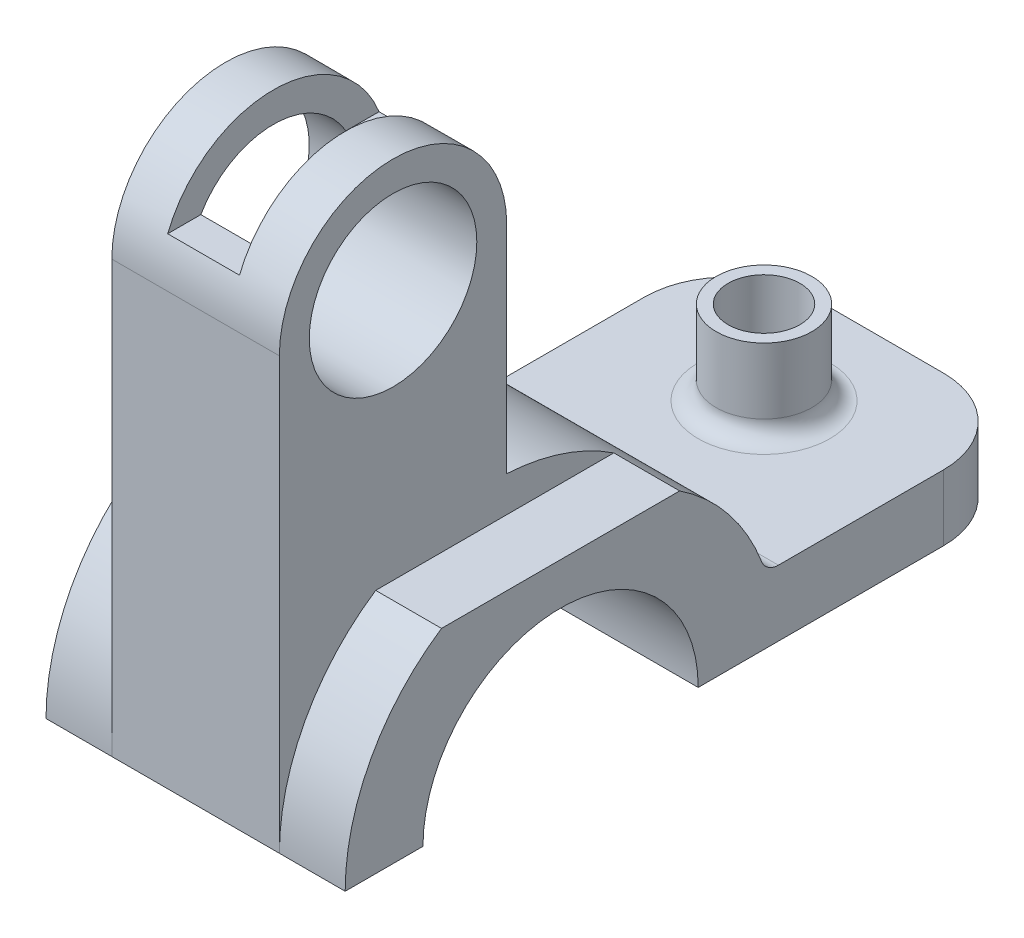
ISO-10303-21;
HEADER;
FILE_DESCRIPTION(('STEP AP214'),'2;1');
FILE_NAME('part.step','',(''),(''),'','','');
FILE_SCHEMA(('AUTOMOTIVE_DESIGN { 1 0 10303 214 1 1 1 1 }'));
ENDSEC;
DATA;
#1=APPLICATION_CONTEXT('core data for automotive mechanical design processes');
#2=APPLICATION_PROTOCOL_DEFINITION('international standard','automotive_design',2000,#1);
#3=PRODUCT_CONTEXT('',#1,'mechanical');
#4=PRODUCT('Part','Part','',(#3));
#5=PRODUCT_RELATED_PRODUCT_CATEGORY('part','',(#4));
#6=PRODUCT_DEFINITION_FORMATION('','',#4);
#7=PRODUCT_DEFINITION_CONTEXT('part definition',#1,'design');
#8=PRODUCT_DEFINITION('design','',#6,#7);
#9=PRODUCT_DEFINITION_SHAPE('','',#8);
#10=(LENGTH_UNIT() NAMED_UNIT(*) SI_UNIT(.MILLI.,.METRE.));
#11=(NAMED_UNIT(*) PLANE_ANGLE_UNIT() SI_UNIT($,.RADIAN.));
#12=(NAMED_UNIT(*) SI_UNIT($,.STERADIAN.) SOLID_ANGLE_UNIT());
#13=UNCERTAINTY_MEASURE_WITH_UNIT(LENGTH_MEASURE(1.E-05),#10,'distance_accuracy_value','');
#14=(GEOMETRIC_REPRESENTATION_CONTEXT(3) GLOBAL_UNCERTAINTY_ASSIGNED_CONTEXT((#13)) GLOBAL_UNIT_ASSIGNED_CONTEXT((#10,
#11,#12)) REPRESENTATION_CONTEXT('',''));
#15=CARTESIAN_POINT('',(0.,0.,0.));
#16=DIRECTION('',(0.,0.,1.));
#17=DIRECTION('',(1.,0.,0.));
#18=AXIS2_PLACEMENT_3D('',#15,#16,#17);
#19=CARTESIAN_POINT('',(14.,72.,17.));
#20=DIRECTION('',(-1.,0.,0.));
#21=DIRECTION('',(0.,0.,1.));
#22=AXIS2_PLACEMENT_3D('',#19,#20,#21);
#23=CYLINDRICAL_SURFACE('',#22,19.);
#24=CARTESIAN_POINT('',(14.,72.,17.));
#25=DIRECTION('',(1.,0.,0.));
#26=DIRECTION('',(0.,0.,-1.));
#27=AXIS2_PLACEMENT_3D('',#24,#25,#26);
#28=CIRCLE('',#27,19.);
#29=CARTESIAN_POINT('',(14.,72.,-1.99999999999999));
#30=VERTEX_POINT('',#29);
#31=CARTESIAN_POINT('',(14.,72.,36.));
#32=VERTEX_POINT('',#31);
#33=EDGE_CURVE('E308',#30,#32,#28,.T.);
#34=ORIENTED_EDGE('',*,*,#33,.F.);
#35=DIRECTION('',(-1.,0.,0.));
#36=VECTOR('',#35,1.);
#37=CARTESIAN_POINT('',(14.,72.,-1.99999999999999));
#38=LINE('',#37,#36);
#39=CARTESIAN_POINT('',(-14.,72.,-1.99999999999999));
#40=VERTEX_POINT('',#39);
#41=EDGE_CURVE('E288',#30,#40,#38,.T.);
#42=ORIENTED_EDGE('',*,*,#41,.T.);
#43=CARTESIAN_POINT('',(-14.,72.,17.));
#44=DIRECTION('',(1.,0.,0.));
#45=DIRECTION('',(0.,0.,-1.));
#46=AXIS2_PLACEMENT_3D('',#43,#44,#45);
#47=CIRCLE('',#46,19.);
#48=CARTESIAN_POINT('',(-14.,72.,36.));
#49=VERTEX_POINT('',#48);
#50=EDGE_CURVE('E314',#40,#49,#47,.T.);
#51=ORIENTED_EDGE('',*,*,#50,.T.);
#52=DIRECTION('',(-1.,0.,0.));
#53=VECTOR('',#52,1.);
#54=CARTESIAN_POINT('',(14.,72.,36.));
#55=LINE('',#54,#53);
#56=EDGE_CURVE('E293',#32,#49,#55,.T.);
#57=ORIENTED_EDGE('',*,*,#56,.F.);
#58=EDGE_LOOP('',(#34,#42,#51,#57));
#59=FACE_BOUND('',#58,.T.);
#60=CARTESIAN_POINT('',(-6.,72.,17.));
#61=DIRECTION('',(1.,0.,0.));
#62=DIRECTION('',(0.,0.,-1.));
#63=AXIS2_PLACEMENT_3D('',#60,#61,#62);
#64=CIRCLE('',#63,19.);
#65=CARTESIAN_POINT('',(-6.,78.9999999999999,-0.663521732655735));
#66=VERTEX_POINT('',#65);
#67=CARTESIAN_POINT('',(-6.,78.9999999999997,34.6635217326558));
#68=VERTEX_POINT('',#67);
#69=EDGE_CURVE('E53',#66,#68,#64,.T.);
#70=ORIENTED_EDGE('',*,*,#69,.F.);
#71=DIRECTION('',(-1.,0.,0.));
#72=VECTOR('',#71,1.);
#73=CARTESIAN_POINT('',(14.,78.9999999999999,-0.663521732655735));
#74=LINE('',#73,#72);
#75=CARTESIAN_POINT('',(6.,78.9999999999999,-0.663521732655735));
#76=VERTEX_POINT('',#75);
#77=EDGE_CURVE('E354',#76,#66,#74,.T.);
#78=ORIENTED_EDGE('',*,*,#77,.F.);
#79=CARTESIAN_POINT('',(6.,72.,17.));
#80=DIRECTION('',(-1.,0.,0.));
#81=DIRECTION('',(0.,0.,1.));
#82=AXIS2_PLACEMENT_3D('',#79,#80,#81);
#83=CIRCLE('',#82,19.);
#84=CARTESIAN_POINT('',(6.,78.9999999999997,34.6635217326558));
#85=VERTEX_POINT('',#84);
#86=EDGE_CURVE('E348',#85,#76,#83,.T.);
#87=ORIENTED_EDGE('',*,*,#86,.F.);
#88=DIRECTION('',(-1.,0.,0.));
#89=VECTOR('',#88,1.);
#90=CARTESIAN_POINT('',(14.,78.9999999999997,34.6635217326558));
#91=LINE('',#90,#89);
#92=EDGE_CURVE('E355',#68,#85,#91,.F.);
#93=ORIENTED_EDGE('',*,*,#92,.F.);
#94=EDGE_LOOP('',(#70,#78,#87,#93));
#95=FACE_BOUND('',#94,.T.);
#96=ADVANCED_FACE('F39',(#59,#95),#23,.T.);
#97=CARTESIAN_POINT('',(25.,72.,17.));
#98=DIRECTION('',(-1.,0.,0.));
#99=DIRECTION('',(0.,0.,1.));
#100=AXIS2_PLACEMENT_3D('',#97,#98,#99);
#101=CYLINDRICAL_SURFACE('',#100,14.);
#102=CARTESIAN_POINT('',(-14.,72.,17.));
#103=DIRECTION('',(-1.,0.,0.));
#104=DIRECTION('',(0.,0.,1.));
#105=AXIS2_PLACEMENT_3D('',#102,#103,#104);
#106=CIRCLE('',#105,14.);
#107=CARTESIAN_POINT('',(-14.,72.,31.));
#108=VERTEX_POINT('',#107);
#109=EDGE_CURVE('E325',#108,#108,#106,.T.);
#110=ORIENTED_EDGE('',*,*,#109,.T.);
#111=EDGE_LOOP('',(#110));
#112=FACE_BOUND('',#111,.T.);
#113=CARTESIAN_POINT('',(14.,72.,17.));
#114=DIRECTION('',(1.,0.,0.));
#115=DIRECTION('',(0.,0.,-1.));
#116=AXIS2_PLACEMENT_3D('',#113,#114,#115);
#117=CIRCLE('',#116,14.);
#118=CARTESIAN_POINT('',(14.,72.,3.00000000000001));
#119=VERTEX_POINT('',#118);
#120=EDGE_CURVE('E320',#119,#119,#117,.T.);
#121=ORIENTED_EDGE('',*,*,#120,.T.);
#122=EDGE_LOOP('',(#121));
#123=FACE_BOUND('',#122,.T.);
#124=DIRECTION('',(-1.,0.,0.));
#125=VECTOR('',#124,1.);
#126=CARTESIAN_POINT('',(25.,78.9999999999999,4.87564434701779));
#127=LINE('',#126,#125);
#128=CARTESIAN_POINT('',(-6.,78.9999999999999,4.87564434701779));
#129=VERTEX_POINT('',#128);
#130=CARTESIAN_POINT('',(6.,78.9999999999999,4.87564434701779));
#131=VERTEX_POINT('',#130);
#132=EDGE_CURVE('E11',#129,#131,#127,.F.);
#133=ORIENTED_EDGE('',*,*,#132,.F.);
#134=CARTESIAN_POINT('',(-6.,72.,17.));
#135=DIRECTION('',(1.,0.,0.));
#136=DIRECTION('',(0.,0.,-1.));
#137=AXIS2_PLACEMENT_3D('',#134,#135,#136);
#138=CIRCLE('',#137,14.);
#139=CARTESIAN_POINT('',(-6.,78.9999999999998,29.1243556529823));
#140=VERTEX_POINT('',#139);
#141=EDGE_CURVE('E50',#140,#129,#138,.F.);
#142=ORIENTED_EDGE('',*,*,#141,.F.);
#143=DIRECTION('',(-1.,0.,0.));
#144=VECTOR('',#143,1.);
#145=CARTESIAN_POINT('',(25.,78.9999999999998,29.1243556529823));
#146=LINE('',#145,#144);
#147=CARTESIAN_POINT('',(6.,78.9999999999998,29.1243556529823));
#148=VERTEX_POINT('',#147);
#149=EDGE_CURVE('E181',#148,#140,#146,.T.);
#150=ORIENTED_EDGE('',*,*,#149,.F.);
#151=CARTESIAN_POINT('',(6.,72.,17.));
#152=DIRECTION('',(-1.,0.,0.));
#153=DIRECTION('',(0.,0.,1.));
#154=AXIS2_PLACEMENT_3D('',#151,#152,#153);
#155=CIRCLE('',#154,14.);
#156=EDGE_CURVE('E189',#131,#148,#155,.F.);
#157=ORIENTED_EDGE('',*,*,#156,.F.);
#158=EDGE_LOOP('',(#133,#142,#150,#157));
#159=FACE_BOUND('',#158,.T.);
#160=ADVANCED_FACE('F196',(#112,#123,#159),#101,.F.);
#161=CARTESIAN_POINT('',(25.,0.,0.));
#162=DIRECTION('',(-1.,0.,0.));
#163=DIRECTION('',(0.,0.,1.));
#164=AXIS2_PLACEMENT_3D('',#161,#162,#163);
#165=CYLINDRICAL_SURFACE('',#164,36.);
#166=CARTESIAN_POINT('',(25.,0.,0.));
#167=DIRECTION('',(1.,0.,0.));
#168=DIRECTION('',(0.,0.,-1.));
#169=AXIS2_PLACEMENT_3D('',#166,#167,#168);
#170=CIRCLE('',#169,36.);
#171=CARTESIAN_POINT('',(25.,30.,19.8997487421324));
#172=VERTEX_POINT('',#171);
#173=CARTESIAN_POINT('',(25.,-2.51386656396706E-13,36.));
#174=VERTEX_POINT('',#173);
#175=EDGE_CURVE('E268',#172,#174,#170,.T.);
#176=ORIENTED_EDGE('',*,*,#175,.F.);
#177=DIRECTION('',(1.,0.,0.));
#178=VECTOR('',#177,1.);
#179=CARTESIAN_POINT('',(-26.2492235949962,30.,19.8997487421324));
#180=LINE('',#179,#178);
#181=CARTESIAN_POINT('',(14.,30.,19.8997487421324));
#182=VERTEX_POINT('',#181);
#183=EDGE_CURVE('E339',#182,#172,#180,.T.);
#184=ORIENTED_EDGE('',*,*,#183,.F.);
#185=CARTESIAN_POINT('',(14.,0.,0.));
#186=DIRECTION('',(-1.,0.,0.));
#187=DIRECTION('',(0.,0.,-1.));
#188=AXIS2_PLACEMENT_3D('',#185,#186,#187);
#189=CIRCLE('',#188,36.);
#190=CARTESIAN_POINT('',(14.,-2.51386656396706E-13,36.));
#191=VERTEX_POINT('',#190);
#192=EDGE_CURVE('E301',#191,#182,#189,.T.);
#193=ORIENTED_EDGE('',*,*,#192,.F.);
#194=DIRECTION('',(-1.,0.,0.));
#195=VECTOR('',#194,1.);
#196=CARTESIAN_POINT('',(25.,-2.51386656396706E-13,36.));
#197=LINE('',#196,#195);
#198=EDGE_CURVE('E239',#174,#191,#197,.T.);
#199=ORIENTED_EDGE('',*,*,#198,.F.);
#200=EDGE_LOOP('',(#176,#184,#193,#199));
#201=FACE_BOUND('',#200,.T.);
#202=ADVANCED_FACE('F378',(#201),#165,.T.);
#203=CARTESIAN_POINT('',(-14.,0.,0.));
#204=DIRECTION('',(-1.,0.,0.));
#205=DIRECTION('',(0.,0.,-1.));
#206=AXIS2_PLACEMENT_3D('',#203,#204,#205);
#207=CIRCLE('',#206,36.);
#208=CARTESIAN_POINT('',(-14.,-2.51386656396706E-13,36.));
#209=VERTEX_POINT('',#208);
#210=CARTESIAN_POINT('',(-14.,30.,19.8997487421324));
#211=VERTEX_POINT('',#210);
#212=EDGE_CURVE('E304',#209,#211,#207,.T.);
#213=ORIENTED_EDGE('',*,*,#212,.T.);
#214=DIRECTION('',(-1.,0.,0.));
#215=VECTOR('',#214,1.);
#216=CARTESIAN_POINT('',(26.2492235949962,30.,19.8997487421324));
#217=LINE('',#216,#215);
#218=CARTESIAN_POINT('',(-25.,30.,19.8997487421324));
#219=VERTEX_POINT('',#218);
#220=EDGE_CURVE('E327',#211,#219,#217,.T.);
#221=ORIENTED_EDGE('',*,*,#220,.T.);
#222=CARTESIAN_POINT('',(-25.,0.,0.));
#223=DIRECTION('',(1.,0.,0.));
#224=DIRECTION('',(0.,0.,-1.));
#225=AXIS2_PLACEMENT_3D('',#222,#223,#224);
#226=CIRCLE('',#225,36.);
#227=CARTESIAN_POINT('',(-25.,-2.51386656396706E-13,36.));
#228=VERTEX_POINT('',#227);
#229=EDGE_CURVE('E251',#219,#228,#226,.T.);
#230=ORIENTED_EDGE('',*,*,#229,.T.);
#231=EDGE_CURVE('E243',#209,#228,#197,.T.);
#232=ORIENTED_EDGE('',*,*,#231,.F.);
#233=EDGE_LOOP('',(#213,#221,#230,#232));
#234=FACE_BOUND('',#233,.T.);
#235=ADVANCED_FACE('F433',(#234),#165,.T.);
#236=CARTESIAN_POINT('',(25.,0.,0.));
#237=DIRECTION('',(-1.,0.,0.));
#238=DIRECTION('',(0.,0.,1.));
#239=AXIS2_PLACEMENT_3D('',#236,#237,#238);
#240=CYLINDRICAL_SURFACE('',#239,23.);
#241=CARTESIAN_POINT('',(-25.,0.,0.));
#242=DIRECTION('',(-1.,0.,0.));
#243=DIRECTION('',(0.,0.,-1.));
#244=AXIS2_PLACEMENT_3D('',#241,#242,#243);
#245=CIRCLE('',#244,23.);
#246=CARTESIAN_POINT('',(-25.,-2.05997398991745E-13,23.));
#247=VERTEX_POINT('',#246);
#248=CARTESIAN_POINT('',(-25.,0.,-23.));
#249=VERTEX_POINT('',#248);
#250=EDGE_CURVE('E261',#247,#249,#245,.T.);
#251=ORIENTED_EDGE('',*,*,#250,.T.);
#252=DIRECTION('',(-1.,0.,0.));
#253=VECTOR('',#252,1.);
#254=CARTESIAN_POINT('',(25.,0.,-23.));
#255=LINE('',#254,#253);
#256=CARTESIAN_POINT('',(25.,0.,-23.));
#257=VERTEX_POINT('',#256);
#258=EDGE_CURVE('E233',#257,#249,#255,.T.);
#259=ORIENTED_EDGE('',*,*,#258,.F.);
#260=CARTESIAN_POINT('',(25.,0.,0.));
#261=DIRECTION('',(-1.,0.,0.));
#262=DIRECTION('',(0.,0.,-1.));
#263=AXIS2_PLACEMENT_3D('',#260,#261,#262);
#264=CIRCLE('',#263,23.);
#265=CARTESIAN_POINT('',(25.,-2.05997398991745E-13,23.));
#266=VERTEX_POINT('',#265);
#267=EDGE_CURVE('E249',#266,#257,#264,.T.);
#268=ORIENTED_EDGE('',*,*,#267,.F.);
#269=DIRECTION('',(-1.,0.,0.));
#270=VECTOR('',#269,1.);
#271=CARTESIAN_POINT('',(25.,-2.05997398991745E-13,23.));
#272=LINE('',#271,#270);
#273=EDGE_CURVE('E242',#266,#247,#272,.T.);
#274=ORIENTED_EDGE('',*,*,#273,.T.);
#275=EDGE_LOOP('',(#251,#259,#268,#274));
#276=FACE_BOUND('',#275,.T.);
#277=ADVANCED_FACE('F443',(#276),#240,.F.);
#278=CARTESIAN_POINT('',(25.,0.,-23.));
#279=DIRECTION('',(0.,1.,0.));
#280=DIRECTION('',(0.,0.,1.));
#281=AXIS2_PLACEMENT_3D('',#278,#279,#280);
#282=PLANE('',#281);
#283=CARTESIAN_POINT('',(0.,-2.53269627492614E-13,-59.));
#284=DIRECTION('',(0.,1.,0.));
#285=DIRECTION('',(0.,0.,1.));
#286=AXIS2_PLACEMENT_3D('',#283,#284,#285);
#287=CIRCLE('',#286,6.);
#288=CARTESIAN_POINT('',(0.,-2.53983803823503E-13,-53.));
#289=VERTEX_POINT('',#288);
#290=EDGE_CURVE('E278',#289,#289,#287,.T.);
#291=ORIENTED_EDGE('',*,*,#290,.T.);
#292=EDGE_LOOP('',(#291));
#293=FACE_BOUND('',#292,.T.);
#294=DIRECTION('',(-1.,0.,0.));
#295=VECTOR('',#294,1.);
#296=CARTESIAN_POINT('',(25.,0.,-78.));
#297=LINE('',#296,#295);
#298=CARTESIAN_POINT('',(11.,0.,-78.));
#299=VERTEX_POINT('',#298);
#300=CARTESIAN_POINT('',(-11.,0.,-78.));
#301=VERTEX_POINT('',#300);
#302=EDGE_CURVE('E234',#299,#301,#297,.T.);
#303=ORIENTED_EDGE('',*,*,#302,.F.);
#304=CARTESIAN_POINT('',(11.,0.,-64.));
#305=DIRECTION('',(0.,1.,0.));
#306=DIRECTION('',(0.,0.,1.));
#307=AXIS2_PLACEMENT_3D('',#304,#305,#306);
#308=CIRCLE('',#307,14.);
#309=CARTESIAN_POINT('',(25.,0.,-64.));
#310=VERTEX_POINT('',#309);
#311=EDGE_CURVE('E213',#299,#310,#308,.F.);
#312=ORIENTED_EDGE('',*,*,#311,.T.);
#313=DIRECTION('',(0.,0.,-1.));
#314=VECTOR('',#313,1.);
#315=CARTESIAN_POINT('',(25.,0.,-23.));
#316=LINE('',#315,#314);
#317=EDGE_CURVE('E271',#257,#310,#316,.T.);
#318=ORIENTED_EDGE('',*,*,#317,.F.);
#319=ORIENTED_EDGE('',*,*,#258,.T.);
#320=DIRECTION('',(0.,0.,-1.));
#321=VECTOR('',#320,1.);
#322=CARTESIAN_POINT('',(-25.,0.,-23.));
#323=LINE('',#322,#321);
#324=CARTESIAN_POINT('',(-25.,0.,-64.));
#325=VERTEX_POINT('',#324);
#326=EDGE_CURVE('E259',#249,#325,#323,.T.);
#327=ORIENTED_EDGE('',*,*,#326,.T.);
#328=CARTESIAN_POINT('',(-11.,0.,-64.));
#329=DIRECTION('',(0.,1.,0.));
#330=DIRECTION('',(0.,0.,1.));
#331=AXIS2_PLACEMENT_3D('',#328,#329,#330);
#332=CIRCLE('',#331,14.);
#333=EDGE_CURVE('E220',#325,#301,#332,.F.);
#334=ORIENTED_EDGE('',*,*,#333,.T.);
#335=EDGE_LOOP('',(#303,#312,#318,#319,#327,#334));
#336=FACE_BOUND('',#335,.T.);
#337=ADVANCED_FACE('F439',(#293,#336),#282,.F.);
#338=CARTESIAN_POINT('',(25.,0.,-78.));
#339=DIRECTION('',(0.,0.,1.));
#340=DIRECTION('',(1.,0.,0.));
#341=AXIS2_PLACEMENT_3D('',#338,#339,#340);
#342=PLANE('',#341);
#343=DIRECTION('',(-1.,0.,0.));
#344=VECTOR('',#343,1.);
#345=CARTESIAN_POINT('',(25.,11.,-78.));
#346=LINE('',#345,#344);
#347=CARTESIAN_POINT('',(11.,11.,-78.));
#348=VERTEX_POINT('',#347);
#349=CARTESIAN_POINT('',(-11.,11.,-78.));
#350=VERTEX_POINT('',#349);
#351=EDGE_CURVE('E240',#348,#350,#346,.T.);
#352=ORIENTED_EDGE('',*,*,#351,.F.);
#353=DIRECTION('',(0.,1.,0.));
#354=VECTOR('',#353,1.);
#355=CARTESIAN_POINT('',(11.,0.,-78.));
#356=LINE('',#355,#354);
#357=EDGE_CURVE('E218',#348,#299,#356,.F.);
#358=ORIENTED_EDGE('',*,*,#357,.T.);
#359=ORIENTED_EDGE('',*,*,#302,.T.);
#360=DIRECTION('',(0.,1.,0.));
#361=VECTOR('',#360,1.);
#362=CARTESIAN_POINT('',(-11.,0.,-78.));
#363=LINE('',#362,#361);
#364=EDGE_CURVE('E224',#301,#350,#363,.T.);
#365=ORIENTED_EDGE('',*,*,#364,.T.);
#366=EDGE_LOOP('',(#352,#358,#359,#365));
#367=FACE_BOUND('',#366,.T.);
#368=ADVANCED_FACE('F436',(#367),#342,.F.);
#369=CARTESIAN_POINT('',(25.,11.,-78.));
#370=DIRECTION('',(0.,-1.,0.));
#371=DIRECTION('',(0.,0.,-1.));
#372=AXIS2_PLACEMENT_3D('',#369,#370,#371);
#373=PLANE('',#372);
#374=CARTESIAN_POINT('',(0.,11.,-59.));
#375=DIRECTION('',(0.,-1.,0.));
#376=DIRECTION('',(0.,0.,-1.));
#377=AXIS2_PLACEMENT_3D('',#374,#375,#376);
#378=CIRCLE('',#377,11.);
#379=CARTESIAN_POINT('',(0.,11.,-70.));
#380=VERTEX_POINT('',#379);
#381=EDGE_CURVE('E210',#380,#380,#378,.T.);
#382=ORIENTED_EDGE('',*,*,#381,.T.);
#383=EDGE_LOOP('',(#382));
#384=FACE_BOUND('',#383,.T.);
#385=DIRECTION('',(0.,0.,1.));
#386=VECTOR('',#385,1.);
#387=CARTESIAN_POINT('',(-25.,11.,-78.));
#388=LINE('',#387,#386);
#389=CARTESIAN_POINT('',(-25.,11.,-64.));
#390=VERTEX_POINT('',#389);
#391=CARTESIAN_POINT('',(-25.,11.,-36.4005494464026));
#392=VERTEX_POINT('',#391);
#393=EDGE_CURVE('E253',#390,#392,#388,.T.);
#394=ORIENTED_EDGE('',*,*,#393,.T.);
#395=DIRECTION('',(1.,0.,0.));
#396=VECTOR('',#395,1.);
#397=CARTESIAN_POINT('',(25.,11.,-36.4005494464026));
#398=LINE('',#397,#396);
#399=CARTESIAN_POINT('',(25.,11.,-36.4005494464026));
#400=VERTEX_POINT('',#399);
#401=EDGE_CURVE('E202',#392,#400,#398,.T.);
#402=ORIENTED_EDGE('',*,*,#401,.T.);
#403=DIRECTION('',(0.,0.,1.));
#404=VECTOR('',#403,1.);
#405=CARTESIAN_POINT('',(25.,11.,-78.));
#406=LINE('',#405,#404);
#407=CARTESIAN_POINT('',(25.,11.,-64.));
#408=VERTEX_POINT('',#407);
#409=EDGE_CURVE('E267',#408,#400,#406,.T.);
#410=ORIENTED_EDGE('',*,*,#409,.F.);
#411=CARTESIAN_POINT('',(11.,11.,-64.));
#412=DIRECTION('',(0.,-1.,0.));
#413=DIRECTION('',(0.,0.,-1.));
#414=AXIS2_PLACEMENT_3D('',#411,#412,#413);
#415=CIRCLE('',#414,14.);
#416=EDGE_CURVE('E223',#408,#348,#415,.F.);
#417=ORIENTED_EDGE('',*,*,#416,.T.);
#418=ORIENTED_EDGE('',*,*,#351,.T.);
#419=CARTESIAN_POINT('',(-11.,11.,-64.));
#420=DIRECTION('',(0.,-1.,0.));
#421=DIRECTION('',(0.,0.,-1.));
#422=AXIS2_PLACEMENT_3D('',#419,#420,#421);
#423=CIRCLE('',#422,14.);
#424=EDGE_CURVE('E228',#350,#390,#423,.F.);
#425=ORIENTED_EDGE('',*,*,#424,.T.);
#426=EDGE_LOOP('',(#394,#402,#410,#417,#418,#425));
#427=FACE_BOUND('',#426,.T.);
#428=ADVANCED_FACE('F431',(#384,#427),#373,.F.);
#429=CARTESIAN_POINT('',(14.,0.,0.));
#430=DIRECTION('',(1.,0.,0.));
#431=DIRECTION('',(0.,0.,-1.));
#432=AXIS2_PLACEMENT_3D('',#429,#430,#431);
#433=CIRCLE('',#432,36.);
#434=CARTESIAN_POINT('',(14.,35.9444015112229,-1.99999999999999));
#435=VERTEX_POINT('',#434);
#436=CARTESIAN_POINT('',(14.,30.,-19.8997487421324));
#437=VERTEX_POINT('',#436);
#438=EDGE_CURVE('E336',#435,#437,#433,.F.);
#439=ORIENTED_EDGE('',*,*,#438,.T.);
#440=DIRECTION('',(1.,0.,0.));
#441=VECTOR('',#440,1.);
#442=CARTESIAN_POINT('',(-26.2492235949962,30.,-19.8997487421324));
#443=LINE('',#442,#441);
#444=CARTESIAN_POINT('',(25.,30.,-19.8997487421324));
#445=VERTEX_POINT('',#444);
#446=EDGE_CURVE('E342',#437,#445,#443,.T.);
#447=ORIENTED_EDGE('',*,*,#446,.T.);
#448=CARTESIAN_POINT('',(25.,12.9230769230769,-33.6005071812947));
#449=VERTEX_POINT('',#448);
#450=EDGE_CURVE('E269',#449,#445,#170,.T.);
#451=ORIENTED_EDGE('',*,*,#450,.F.);
#452=DIRECTION('',(-1.,0.,0.));
#453=VECTOR('',#452,1.);
#454=CARTESIAN_POINT('',(25.,12.9230769230769,-33.6005071812947));
#455=LINE('',#454,#453);
#456=CARTESIAN_POINT('',(-25.,12.9230769230769,-33.6005071812947));
#457=VERTEX_POINT('',#456);
#458=EDGE_CURVE('E208',#449,#457,#455,.T.);
#459=ORIENTED_EDGE('',*,*,#458,.T.);
#460=CARTESIAN_POINT('',(-25.,30.,-19.8997487421324));
#461=VERTEX_POINT('',#460);
#462=EDGE_CURVE('E252',#457,#461,#226,.T.);
#463=ORIENTED_EDGE('',*,*,#462,.T.);
#464=DIRECTION('',(-1.,0.,0.));
#465=VECTOR('',#464,1.);
#466=CARTESIAN_POINT('',(26.2492235949962,30.,-19.8997487421324));
#467=LINE('',#466,#465);
#468=CARTESIAN_POINT('',(-14.,30.,-19.8997487421324));
#469=VERTEX_POINT('',#468);
#470=EDGE_CURVE('E323',#469,#461,#467,.T.);
#471=ORIENTED_EDGE('',*,*,#470,.F.);
#472=CARTESIAN_POINT('',(-14.,-1.11022302462516E-13,0.));
#473=DIRECTION('',(1.,0.,0.));
#474=DIRECTION('',(0.,0.,-1.));
#475=AXIS2_PLACEMENT_3D('',#472,#473,#474);
#476=CIRCLE('',#475,36.0000000000001);
#477=CARTESIAN_POINT('',(-14.,35.9444015112228,-1.99999999999999));
#478=VERTEX_POINT('',#477);
#479=EDGE_CURVE('E330',#478,#469,#476,.F.);
#480=ORIENTED_EDGE('',*,*,#479,.F.);
#481=DIRECTION('',(-1.,0.,0.));
#482=VECTOR('',#481,1.);
#483=CARTESIAN_POINT('',(14.,35.9444015112229,-1.99999999999999));
#484=LINE('',#483,#482);
#485=EDGE_CURVE('E283',#435,#478,#484,.T.);
#486=ORIENTED_EDGE('',*,*,#485,.F.);
#487=EDGE_LOOP('',(#439,#447,#451,#459,#463,#471,#480,#486));
#488=FACE_BOUND('',#487,.T.);
#489=ADVANCED_FACE('F430',(#488),#165,.T.);
#490=CARTESIAN_POINT('',(25.,-2.05997398991745E-13,23.));
#491=DIRECTION('',(0.,1.,0.));
#492=DIRECTION('',(0.,0.,1.));
#493=AXIS2_PLACEMENT_3D('',#490,#491,#492);
#494=PLANE('',#493);
#495=DIRECTION('',(0.,0.,-1.));
#496=VECTOR('',#495,1.);
#497=CARTESIAN_POINT('',(-25.,-2.05997398991745E-13,23.));
#498=LINE('',#497,#496);
#499=EDGE_CURVE('E247',#228,#247,#498,.T.);
#500=ORIENTED_EDGE('',*,*,#499,.T.);
#501=ORIENTED_EDGE('',*,*,#273,.F.);
#502=DIRECTION('',(0.,0.,-1.));
#503=VECTOR('',#502,1.);
#504=CARTESIAN_POINT('',(25.,-2.05997398991745E-13,23.));
#505=LINE('',#504,#503);
#506=EDGE_CURVE('E250',#174,#266,#505,.T.);
#507=ORIENTED_EDGE('',*,*,#506,.F.);
#508=ORIENTED_EDGE('',*,*,#198,.T.);
#509=DIRECTION('',(-1.,0.,0.));
#510=VECTOR('',#509,1.);
#511=CARTESIAN_POINT('',(14.,-2.51386656396706E-13,36.));
#512=LINE('',#511,#510);
#513=EDGE_CURVE('E295',#191,#209,#512,.T.);
#514=ORIENTED_EDGE('',*,*,#513,.T.);
#515=ORIENTED_EDGE('',*,*,#231,.T.);
#516=EDGE_LOOP('',(#500,#501,#507,#508,#514,#515));
#517=FACE_BOUND('',#516,.T.);
#518=ADVANCED_FACE('F418',(#517),#494,.F.);
#519=CARTESIAN_POINT('',(25.,0.,0.));
#520=DIRECTION('',(1.,0.,0.));
#521=DIRECTION('',(0.,0.,-1.));
#522=AXIS2_PLACEMENT_3D('',#519,#520,#521);
#523=PLANE('',#522);
#524=DIRECTION('',(0.,0.,-1.));
#525=VECTOR('',#524,1.);
#526=CARTESIAN_POINT('',(25.,30.,-19.8997487421324));
#527=LINE('',#526,#525);
#528=EDGE_CURVE('E345',#172,#445,#527,.T.);
#529=ORIENTED_EDGE('',*,*,#528,.F.);
#530=ORIENTED_EDGE('',*,*,#175,.T.);
#531=ORIENTED_EDGE('',*,*,#506,.T.);
#532=ORIENTED_EDGE('',*,*,#267,.T.);
#533=ORIENTED_EDGE('',*,*,#317,.T.);
#534=DIRECTION('',(0.,1.,0.));
#535=VECTOR('',#534,1.);
#536=CARTESIAN_POINT('',(25.,11.,-64.));
#537=LINE('',#536,#535);
#538=EDGE_CURVE('E226',#310,#408,#537,.T.);
#539=ORIENTED_EDGE('',*,*,#538,.T.);
#540=ORIENTED_EDGE('',*,*,#409,.T.);
#541=CARTESIAN_POINT('',(25.,14.,-36.4005494464026));
#542=DIRECTION('',(1.,0.,0.));
#543=DIRECTION('',(0.,0.,-1.));
#544=AXIS2_PLACEMENT_3D('',#541,#542,#543);
#545=CIRCLE('',#544,3.);
#546=EDGE_CURVE('E186',#400,#449,#545,.F.);
#547=ORIENTED_EDGE('',*,*,#546,.T.);
#548=ORIENTED_EDGE('',*,*,#450,.T.);
#549=EDGE_LOOP('',(#529,#530,#531,#532,#533,#539,#540,#547,#548));
#550=FACE_BOUND('',#549,.T.);
#551=ADVANCED_FACE('F414',(#550),#523,.T.);
#552=CARTESIAN_POINT('',(-25.,0.,0.));
#553=DIRECTION('',(1.,0.,0.));
#554=DIRECTION('',(0.,0.,-1.));
#555=AXIS2_PLACEMENT_3D('',#552,#553,#554);
#556=PLANE('',#555);
#557=ORIENTED_EDGE('',*,*,#229,.F.);
#558=DIRECTION('',(0.,0.,1.));
#559=VECTOR('',#558,1.);
#560=CARTESIAN_POINT('',(-25.,30.,-19.8997487421324));
#561=LINE('',#560,#559);
#562=EDGE_CURVE('E333',#461,#219,#561,.T.);
#563=ORIENTED_EDGE('',*,*,#562,.F.);
#564=ORIENTED_EDGE('',*,*,#462,.F.);
#565=CARTESIAN_POINT('',(-25.,14.,-36.4005494464026));
#566=DIRECTION('',(1.,0.,0.));
#567=DIRECTION('',(0.,0.,-1.));
#568=AXIS2_PLACEMENT_3D('',#565,#566,#567);
#569=CIRCLE('',#568,3.);
#570=EDGE_CURVE('E199',#457,#392,#569,.T.);
#571=ORIENTED_EDGE('',*,*,#570,.T.);
#572=ORIENTED_EDGE('',*,*,#393,.F.);
#573=DIRECTION('',(0.,1.,0.));
#574=VECTOR('',#573,1.);
#575=CARTESIAN_POINT('',(-25.,0.,-64.));
#576=LINE('',#575,#574);
#577=EDGE_CURVE('E214',#390,#325,#576,.F.);
#578=ORIENTED_EDGE('',*,*,#577,.T.);
#579=ORIENTED_EDGE('',*,*,#326,.F.);
#580=ORIENTED_EDGE('',*,*,#250,.F.);
#581=ORIENTED_EDGE('',*,*,#499,.F.);
#582=EDGE_LOOP('',(#557,#563,#564,#571,#572,#578,#579,#580,#581));
#583=FACE_BOUND('',#582,.T.);
#584=ADVANCED_FACE('F420',(#583),#556,.F.);
#585=CARTESIAN_POINT('',(11.,0.,-64.));
#586=DIRECTION('',(0.,-1.,0.));
#587=DIRECTION('',(0.,0.,-1.));
#588=AXIS2_PLACEMENT_3D('',#585,#586,#587);
#589=CYLINDRICAL_SURFACE('',#588,14.);
#590=ORIENTED_EDGE('',*,*,#311,.F.);
#591=ORIENTED_EDGE('',*,*,#357,.F.);
#592=ORIENTED_EDGE('',*,*,#416,.F.);
#593=ORIENTED_EDGE('',*,*,#538,.F.);
#594=EDGE_LOOP('',(#590,#591,#592,#593));
#595=FACE_BOUND('',#594,.T.);
#596=ADVANCED_FACE('F421',(#595),#589,.T.);
#597=CARTESIAN_POINT('',(-11.,0.,-64.));
#598=DIRECTION('',(0.,1.,0.));
#599=DIRECTION('',(0.,0.,1.));
#600=AXIS2_PLACEMENT_3D('',#597,#598,#599);
#601=CYLINDRICAL_SURFACE('',#600,14.);
#602=ORIENTED_EDGE('',*,*,#333,.F.);
#603=ORIENTED_EDGE('',*,*,#577,.F.);
#604=ORIENTED_EDGE('',*,*,#424,.F.);
#605=ORIENTED_EDGE('',*,*,#364,.F.);
#606=EDGE_LOOP('',(#602,#603,#604,#605));
#607=FACE_BOUND('',#606,.T.);
#608=ADVANCED_FACE('F412',(#607),#601,.T.);
#609=CARTESIAN_POINT('',(0.,25.,-59.));
#610=DIRECTION('',(0.,-1.,0.));
#611=DIRECTION('',(0.,0.,-1.));
#612=AXIS2_PLACEMENT_3D('',#609,#610,#611);
#613=CYLINDRICAL_SURFACE('',#612,8.);
#614=CARTESIAN_POINT('',(0.,14.,-59.));
#615=DIRECTION('',(0.,-1.,0.));
#616=DIRECTION('',(0.,0.,-1.));
#617=AXIS2_PLACEMENT_3D('',#614,#615,#616);
#618=CIRCLE('',#617,8.);
#619=CARTESIAN_POINT('',(0.,14.,-67.));
#620=VERTEX_POINT('',#619);
#621=EDGE_CURVE('E201',#620,#620,#618,.F.);
#622=ORIENTED_EDGE('',*,*,#621,.T.);
#623=EDGE_LOOP('',(#622));
#624=FACE_BOUND('',#623,.T.);
#625=CARTESIAN_POINT('',(0.,25.,-59.));
#626=DIRECTION('',(0.,1.,0.));
#627=DIRECTION('',(0.,0.,1.));
#628=AXIS2_PLACEMENT_3D('',#625,#626,#627);
#629=CIRCLE('',#628,8.);
#630=CARTESIAN_POINT('',(0.,25.,-51.));
#631=VERTEX_POINT('',#630);
#632=EDGE_CURVE('E263',#631,#631,#629,.T.);
#633=ORIENTED_EDGE('',*,*,#632,.F.);
#634=EDGE_LOOP('',(#633));
#635=FACE_BOUND('',#634,.T.);
#636=ADVANCED_FACE('F406',(#624,#635),#613,.T.);
#637=CARTESIAN_POINT('',(0.,25.,-59.));
#638=DIRECTION('',(0.,1.,0.));
#639=DIRECTION('',(0.,0.,1.));
#640=AXIS2_PLACEMENT_3D('',#637,#638,#639);
#641=PLANE('',#640);
#642=CARTESIAN_POINT('',(0.,25.,-59.));
#643=DIRECTION('',(0.,1.,0.));
#644=DIRECTION('',(0.,0.,1.));
#645=AXIS2_PLACEMENT_3D('',#642,#643,#644);
#646=CIRCLE('',#645,6.);
#647=CARTESIAN_POINT('',(0.,25.,-53.));
#648=VERTEX_POINT('',#647);
#649=EDGE_CURVE('E281',#648,#648,#646,.T.);
#650=ORIENTED_EDGE('',*,*,#649,.F.);
#651=EDGE_LOOP('',(#650));
#652=FACE_BOUND('',#651,.T.);
#653=ORIENTED_EDGE('',*,*,#632,.T.);
#654=EDGE_LOOP('',(#653));
#655=FACE_BOUND('',#654,.T.);
#656=ADVANCED_FACE('F403',(#652,#655),#641,.T.);
#657=CARTESIAN_POINT('',(0.,-2.53269627492614E-13,-59.));
#658=DIRECTION('',(0.,1.,0.));
#659=DIRECTION('',(0.,0.,1.));
#660=AXIS2_PLACEMENT_3D('',#657,#658,#659);
#661=CYLINDRICAL_SURFACE('',#660,6.);
#662=ORIENTED_EDGE('',*,*,#290,.F.);
#663=EDGE_LOOP('',(#662));
#664=FACE_BOUND('',#663,.T.);
#665=ORIENTED_EDGE('',*,*,#649,.T.);
#666=EDGE_LOOP('',(#665));
#667=FACE_BOUND('',#666,.T.);
#668=ADVANCED_FACE('F402',(#664,#667),#661,.F.);
#669=CARTESIAN_POINT('',(25.,14.,-36.4005494464026));
#670=DIRECTION('',(-1.,0.,0.));
#671=DIRECTION('',(0.,0.,1.));
#672=AXIS2_PLACEMENT_3D('',#669,#670,#671);
#673=CYLINDRICAL_SURFACE('',#672,3.);
#674=ORIENTED_EDGE('',*,*,#546,.F.);
#675=ORIENTED_EDGE('',*,*,#401,.F.);
#676=ORIENTED_EDGE('',*,*,#570,.F.);
#677=ORIENTED_EDGE('',*,*,#458,.F.);
#678=EDGE_LOOP('',(#674,#675,#676,#677));
#679=FACE_BOUND('',#678,.T.);
#680=ADVANCED_FACE('F404',(#679),#673,.F.);
#681=CARTESIAN_POINT('',(0.,14.,-59.));
#682=DIRECTION('',(0.,-1.,0.));
#683=DIRECTION('',(0.,0.,-1.));
#684=AXIS2_PLACEMENT_3D('',#681,#682,#683);
#685=TOROIDAL_SURFACE('',#684,11.,3.);
#686=ORIENTED_EDGE('',*,*,#381,.F.);
#687=EDGE_LOOP('',(#686));
#688=FACE_BOUND('',#687,.T.);
#689=ORIENTED_EDGE('',*,*,#621,.F.);
#690=EDGE_LOOP('',(#689));
#691=FACE_BOUND('',#690,.T.);
#692=ADVANCED_FACE('F41',(#688,#691),#685,.F.);
#693=CARTESIAN_POINT('',(14.,35.9444015112229,-1.99999999999999));
#694=DIRECTION('',(0.,0.,1.));
#695=DIRECTION('',(1.,0.,0.));
#696=AXIS2_PLACEMENT_3D('',#693,#694,#695);
#697=PLANE('',#696);
#698=DIRECTION('',(0.,1.,0.));
#699=VECTOR('',#698,1.);
#700=CARTESIAN_POINT('',(-14.,35.9444015112229,-1.99999999999999));
#701=LINE('',#700,#699);
#702=EDGE_CURVE('E305',#478,#40,#701,.T.);
#703=ORIENTED_EDGE('',*,*,#702,.T.);
#704=ORIENTED_EDGE('',*,*,#41,.F.);
#705=DIRECTION('',(0.,1.,0.));
#706=VECTOR('',#705,1.);
#707=CARTESIAN_POINT('',(14.,35.9444015112229,-1.99999999999999));
#708=LINE('',#707,#706);
#709=EDGE_CURVE('E309',#435,#30,#708,.T.);
#710=ORIENTED_EDGE('',*,*,#709,.F.);
#711=ORIENTED_EDGE('',*,*,#485,.T.);
#712=EDGE_LOOP('',(#703,#704,#710,#711));
#713=FACE_BOUND('',#712,.T.);
#714=ADVANCED_FACE('F399',(#713),#697,.F.);
#715=CARTESIAN_POINT('',(14.,-2.51386656396706E-13,36.));
#716=DIRECTION('',(0.,0.,-1.));
#717=DIRECTION('',(-1.,0.,0.));
#718=AXIS2_PLACEMENT_3D('',#715,#716,#717);
#719=PLANE('',#718);
#720=DIRECTION('',(0.,-1.,0.));
#721=VECTOR('',#720,1.);
#722=CARTESIAN_POINT('',(-14.,-2.51386656396706E-13,36.));
#723=LINE('',#722,#721);
#724=EDGE_CURVE('E296',#49,#209,#723,.T.);
#725=ORIENTED_EDGE('',*,*,#724,.T.);
#726=ORIENTED_EDGE('',*,*,#513,.F.);
#727=DIRECTION('',(0.,-1.,0.));
#728=VECTOR('',#727,1.);
#729=CARTESIAN_POINT('',(14.,-2.51386656396706E-13,36.));
#730=LINE('',#729,#728);
#731=EDGE_CURVE('E300',#32,#191,#730,.T.);
#732=ORIENTED_EDGE('',*,*,#731,.F.);
#733=ORIENTED_EDGE('',*,*,#56,.T.);
#734=EDGE_LOOP('',(#725,#726,#732,#733));
#735=FACE_BOUND('',#734,.T.);
#736=ADVANCED_FACE('F389',(#735),#719,.F.);
#737=CARTESIAN_POINT('',(14.,0.,0.));
#738=DIRECTION('',(1.,0.,0.));
#739=DIRECTION('',(0.,0.,-1.));
#740=AXIS2_PLACEMENT_3D('',#737,#738,#739);
#741=PLANE('',#740);
#742=ORIENTED_EDGE('',*,*,#120,.F.);
#743=EDGE_LOOP('',(#742));
#744=FACE_BOUND('',#743,.T.);
#745=ORIENTED_EDGE('',*,*,#709,.T.);
#746=ORIENTED_EDGE('',*,*,#33,.T.);
#747=ORIENTED_EDGE('',*,*,#731,.T.);
#748=ORIENTED_EDGE('',*,*,#192,.T.);
#749=DIRECTION('',(0.,0.,1.));
#750=VECTOR('',#749,1.);
#751=CARTESIAN_POINT('',(14.,30.,-19.8997487421324));
#752=LINE('',#751,#750);
#753=EDGE_CURVE('E337',#437,#182,#752,.T.);
#754=ORIENTED_EDGE('',*,*,#753,.F.);
#755=ORIENTED_EDGE('',*,*,#438,.F.);
#756=EDGE_LOOP('',(#745,#746,#747,#748,#754,#755));
#757=FACE_BOUND('',#756,.T.);
#758=ADVANCED_FACE('F381',(#744,#757),#741,.T.);
#759=CARTESIAN_POINT('',(-14.,0.,0.));
#760=DIRECTION('',(1.,0.,0.));
#761=DIRECTION('',(0.,0.,-1.));
#762=AXIS2_PLACEMENT_3D('',#759,#760,#761);
#763=PLANE('',#762);
#764=ORIENTED_EDGE('',*,*,#109,.F.);
#765=EDGE_LOOP('',(#764));
#766=FACE_BOUND('',#765,.T.);
#767=ORIENTED_EDGE('',*,*,#724,.F.);
#768=ORIENTED_EDGE('',*,*,#50,.F.);
#769=ORIENTED_EDGE('',*,*,#702,.F.);
#770=ORIENTED_EDGE('',*,*,#479,.T.);
#771=DIRECTION('',(0.,0.,1.));
#772=VECTOR('',#771,1.);
#773=CARTESIAN_POINT('',(-14.,30.,-19.8997487421324));
#774=LINE('',#773,#772);
#775=EDGE_CURVE('E334',#469,#211,#774,.T.);
#776=ORIENTED_EDGE('',*,*,#775,.T.);
#777=ORIENTED_EDGE('',*,*,#212,.F.);
#778=EDGE_LOOP('',(#767,#768,#769,#770,#776,#777));
#779=FACE_BOUND('',#778,.T.);
#780=ADVANCED_FACE('F390',(#766,#779),#763,.F.);
#781=CARTESIAN_POINT('',(26.2492235949962,30.,-19.8997487421324));
#782=DIRECTION('',(0.,-1.,0.));
#783=DIRECTION('',(0.,0.,-1.));
#784=AXIS2_PLACEMENT_3D('',#781,#782,#783);
#785=PLANE('',#784);
#786=ORIENTED_EDGE('',*,*,#470,.T.);
#787=ORIENTED_EDGE('',*,*,#562,.T.);
#788=ORIENTED_EDGE('',*,*,#220,.F.);
#789=ORIENTED_EDGE('',*,*,#775,.F.);
#790=EDGE_LOOP('',(#786,#787,#788,#789));
#791=FACE_BOUND('',#790,.T.);
#792=ADVANCED_FACE('F395',(#791),#785,.F.);
#793=CARTESIAN_POINT('',(-26.2492235949962,30.,-19.8997487421324));
#794=DIRECTION('',(0.,-1.,0.));
#795=DIRECTION('',(0.,0.,-1.));
#796=AXIS2_PLACEMENT_3D('',#793,#794,#795);
#797=PLANE('',#796);
#798=ORIENTED_EDGE('',*,*,#753,.T.);
#799=ORIENTED_EDGE('',*,*,#183,.T.);
#800=ORIENTED_EDGE('',*,*,#528,.T.);
#801=ORIENTED_EDGE('',*,*,#446,.F.);
#802=EDGE_LOOP('',(#798,#799,#800,#801));
#803=FACE_BOUND('',#802,.T.);
#804=ADVANCED_FACE('F468',(#803),#797,.F.);
#805=CARTESIAN_POINT('',(-6.,78.9999999999999,-1.99999999999984));
#806=DIRECTION('',(1.,0.,0.));
#807=DIRECTION('',(0.,0.,-1.));
#808=AXIS2_PLACEMENT_3D('',#805,#806,#807);
#809=PLANE('',#808);
#810=ORIENTED_EDGE('',*,*,#69,.T.);
#811=DIRECTION('',(0.,0.,-1.));
#812=VECTOR('',#811,1.);
#813=CARTESIAN_POINT('',(-6.,78.9999999999999,-1.99999999999984));
#814=LINE('',#813,#812);
#815=EDGE_CURVE('E182',#68,#140,#814,.T.);
#816=ORIENTED_EDGE('',*,*,#815,.T.);
#817=ORIENTED_EDGE('',*,*,#141,.T.);
#818=EDGE_CURVE('E194',#129,#66,#814,.T.);
#819=ORIENTED_EDGE('',*,*,#818,.T.);
#820=EDGE_LOOP('',(#810,#816,#817,#819));
#821=FACE_BOUND('',#820,.T.);
#822=ADVANCED_FACE('F192',(#821),#809,.T.);
#823=CARTESIAN_POINT('',(6.,78.9999999999999,-1.99999999999984));
#824=DIRECTION('',(-1.,0.,0.));
#825=DIRECTION('',(0.,0.,1.));
#826=AXIS2_PLACEMENT_3D('',#823,#824,#825);
#827=PLANE('',#826);
#828=ORIENTED_EDGE('',*,*,#86,.T.);
#829=DIRECTION('',(0.,0.,1.));
#830=VECTOR('',#829,1.);
#831=CARTESIAN_POINT('',(6.,78.9999999999999,-1.99999999999984));
#832=LINE('',#831,#830);
#833=EDGE_CURVE('E352',#76,#131,#832,.T.);
#834=ORIENTED_EDGE('',*,*,#833,.T.);
#835=ORIENTED_EDGE('',*,*,#156,.T.);
#836=EDGE_CURVE('E65',#148,#85,#832,.T.);
#837=ORIENTED_EDGE('',*,*,#836,.T.);
#838=EDGE_LOOP('',(#828,#834,#835,#837));
#839=FACE_BOUND('',#838,.T.);
#840=ADVANCED_FACE('F363',(#839),#827,.T.);
#841=CARTESIAN_POINT('',(0.,78.9999999999999,2.90438721436808E-13));
#842=DIRECTION('',(0.,1.,0.));
#843=DIRECTION('',(0.,0.,1.));
#844=AXIS2_PLACEMENT_3D('',#841,#842,#843);
#845=PLANE('',#844);
#846=ORIENTED_EDGE('',*,*,#77,.T.);
#847=ORIENTED_EDGE('',*,*,#818,.F.);
#848=ORIENTED_EDGE('',*,*,#132,.T.);
#849=ORIENTED_EDGE('',*,*,#833,.F.);
#850=EDGE_LOOP('',(#846,#847,#848,#849));
#851=FACE_BOUND('',#850,.T.);
#852=ADVANCED_FACE('F364',(#851),#845,.T.);
#853=ORIENTED_EDGE('',*,*,#92,.T.);
#854=ORIENTED_EDGE('',*,*,#836,.F.);
#855=ORIENTED_EDGE('',*,*,#149,.T.);
#856=ORIENTED_EDGE('',*,*,#815,.F.);
#857=EDGE_LOOP('',(#853,#854,#855,#856));
#858=FACE_BOUND('',#857,.T.);
#859=ADVANCED_FACE('F185',(#858),#845,.T.);
#860=CLOSED_SHELL('',(#96,#160,#202,#235,#277,#337,#368,#428,#489,#518,#551,#584,#596,#608,#636,
#656,#668,#680,#692,#714,#736,#758,#780,#792,#804,#822,#840,#852,#859));
#861=MANIFOLD_SOLID_BREP('B2',#860);
#862=ADVANCED_BREP_SHAPE_REPRESENTATION('',(#18,#861),#14);
#863=SHAPE_DEFINITION_REPRESENTATION(#9,#862);
ENDSEC;
END-ISO-10303-21;
